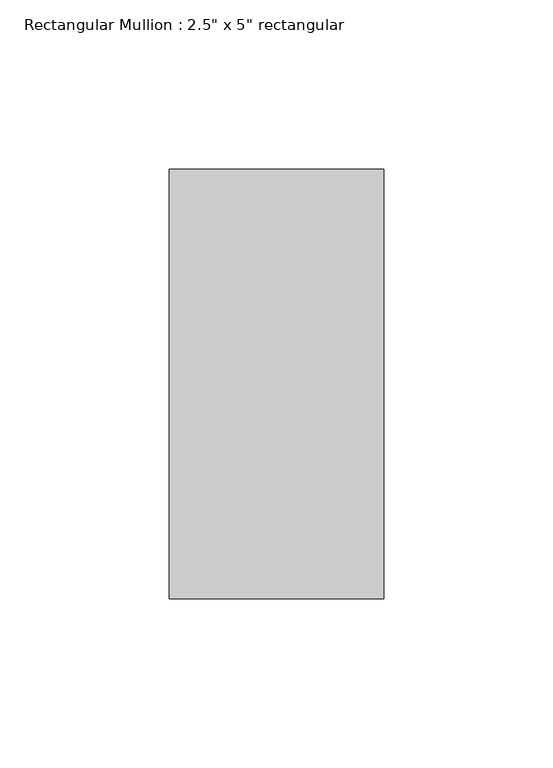
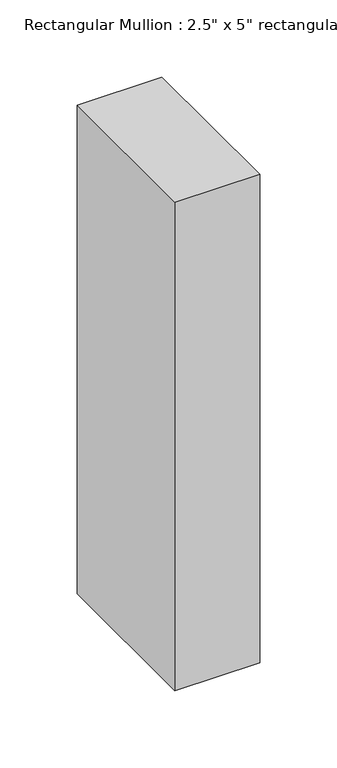
"""IFC4 building model written with IfcOpenShell, lengths in millimetres: member geometry."""

from ifc_helpers import new_model, si_unit, frame, origin, place, context, project, spatial, polyline, outline, extrude, source, transform, mapped, element, save


def member_3709dd30(model_context):
    return source(origin(), model_context, "Body", "SweptSolid", [
        extrude(outline(polyline([(31.75, 63.5), (31.75, -63.5), (-31.75, -63.5), (-31.75, 63.5), (31.75, 63.5)])), frame((0.0, 0.0, -387.35), z_axis=(0.0, 0.0, 1.0), x_axis=(1.0, 0.0, 0.0)), (0.0, 0.0, 1.0), 387.35),
    ])


if __name__ == "__main__":
    model = new_model("IFC4")
    model_context = context("Model", 3, world=origin())
    ifc_project = project(units=[si_unit("LENGTHUNIT", "METRE", prefix="MILLI")], contexts=[model_context])
    site = spatial("IfcSite", under=ifc_project)
    building = spatial("IfcBuilding", under=site)
    placement = place(None, origin())
    member_shape = member_3709dd30(model_context)
    element("IfcMember", 1, ObjectType="Rectangular Mullion : 2.5\" x 5\" rectangular", at=placement, inside=building, context=model_context, shape_type="MappedRepresentation", body=[
        mapped(member_shape, transform((0.0, 0.0, 0.0), x_axis=(1.0, 0.0, 0.0), y_axis=(0.0, 1.0, 0.0), z_axis=(0.0, 0.0, 1.0))),
    ])
    save(model, "model.ifc")

# Revit data of these elements
# Type "Rectangular Mullion : 2.5\" x 5\" rectangular"
#   built-in parameter 1007304 = 0.416667 (stored number, unit not read)
#   built-in parameter 1007301 = 0.104167 (stored number, unit not read)
#   built-in parameter 1007300 = 0.104167 (stored number, unit not read)
# Element 1 (IfcMember, "Rectangular Mullion : 2.5\" x 5\" rectangular")
#   Materials on its faces: "door colour"
# Materials
#   "door colour": class "Generic", colour RGB 120 120 120, transparency 0, Cost = 0
